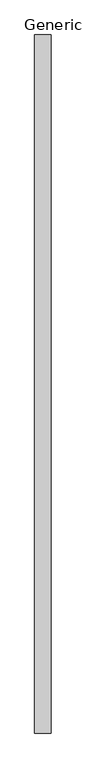
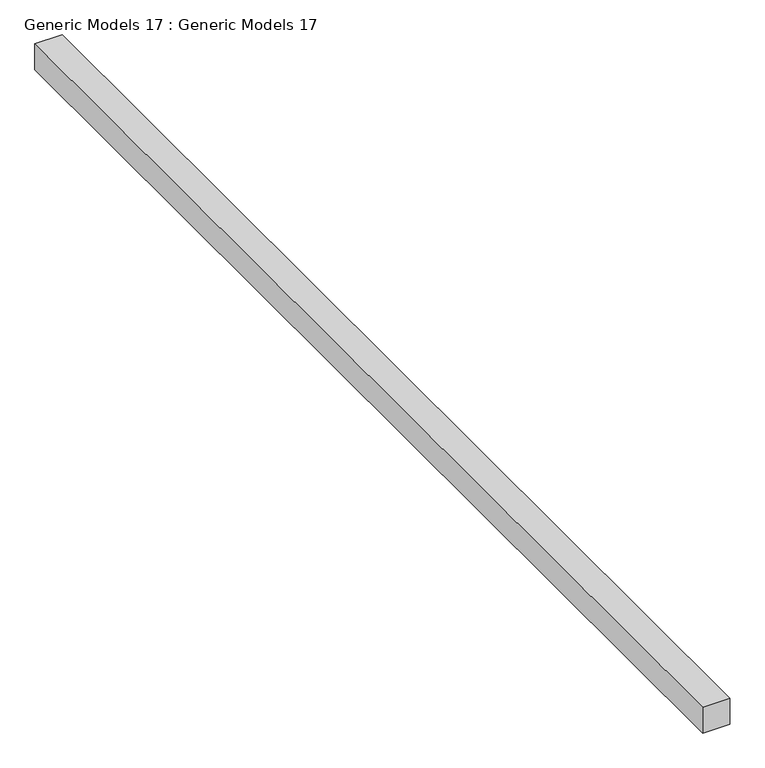
"""IFC4 building model written with IfcOpenShell, lengths in millimetres: proxy geometry, Generic Models 17 : Generic Models 17."""

from ifc_helpers import new_model, si_unit, frame, origin, place, context, project, spatial, polyline, outline, extrude, source, transform, mapped, element, save


def generic_models_17_generic_models_17_16b6177c(model_context):
    return source(origin(), model_context, "Body", "SweptSolid", [
        extrude(outline(polyline([(-15581.438074, -6004.9096639), (-15581.438074, 6878.3014639), (-15276.638074, 6878.3014639), (-15276.638074, -6004.9096639), (-15581.438074, -6004.9096639)])), frame((0.0, 0.0, 22860.0), z_axis=(0.0, 0.0, 1.0), x_axis=(1.0, 0.0, 0.0)), (0.0, 0.0, 1.0), 304.8),
    ])


if __name__ == "__main__":
    model = new_model("IFC4")
    model_context = context("Model", 3, world=origin())
    ifc_project = project(units=[si_unit("LENGTHUNIT", "METRE", prefix="MILLI")], contexts=[model_context])
    site = spatial("IfcSite", under=ifc_project)
    building = spatial("IfcBuilding", under=site)
    placement = place(None, origin())
    generic_models_17_generic_models_17_shape = generic_models_17_generic_models_17_16b6177c(model_context)
    element("IfcBuildingElementProxy", 1, Name="Generic Models 17 : Generic Models 17", ObjectType="Generic Models 17 : Generic Models 17", at=placement, inside=building, context=model_context, shape_type="MappedRepresentation", body=[
        mapped(generic_models_17_generic_models_17_shape, transform((0.0, 0.0, 0.0), x_axis=(1.0, 0.0, 0.0), y_axis=(0.0, 1.0, 0.0), z_axis=(0.0, 0.0, 1.0))),
    ])
    save(model, "model.ifc")
